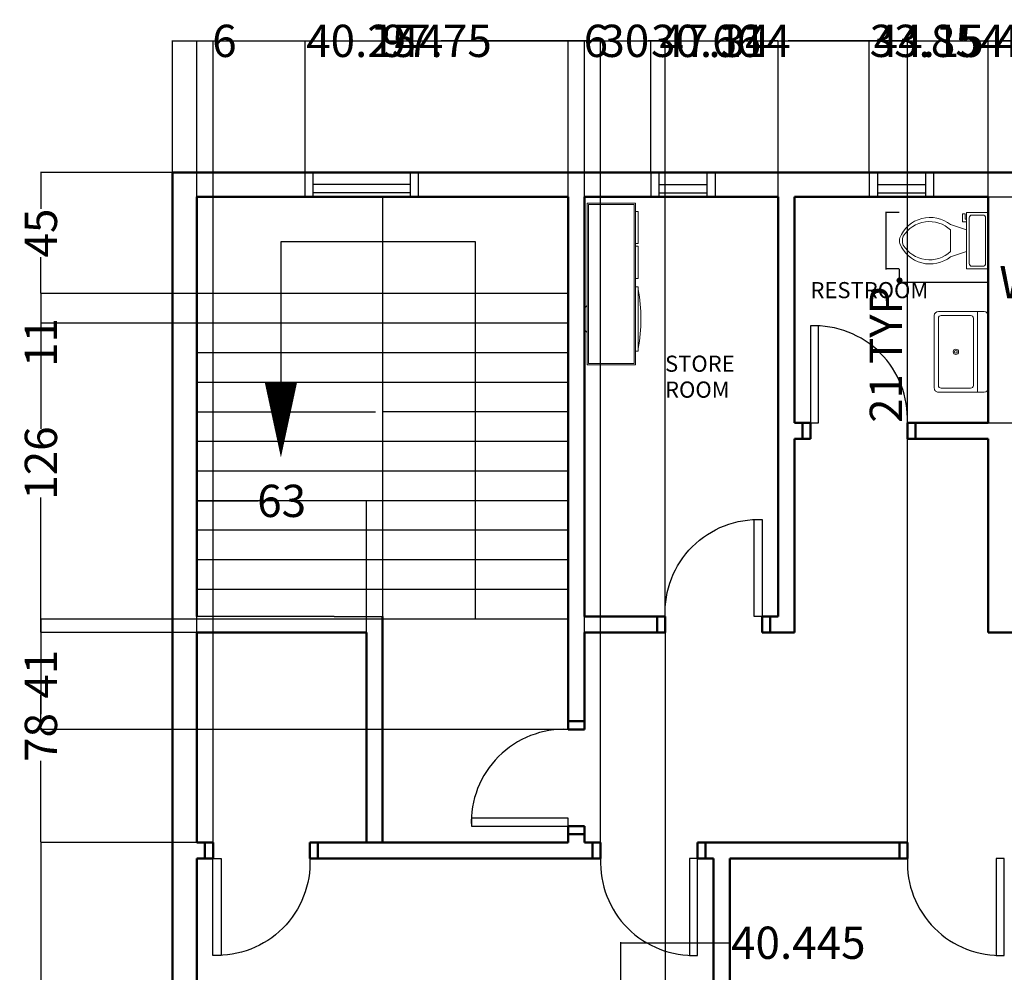
# Model space of a CAD drawing. Units: inches. Extents: x 128 to 1267, y -109 to 1208.
# Tile 6 of 8: x 180 to 546, y 842 to 1196. Entities that reach past the tile are written whole.
import ezdxf

# ---------------------------------------------------------------- set-up
doc = ezdxf.new("R2010")
doc.units = ezdxf.units.IN
doc.header["$MEASUREMENT"] = 0
for name, color, linetype, lineweight in [('A-ANNO-DIMS', 2, 'Continuous', 18), ('A-AREA-IDEN', 3, 'Continuous', 25), ('A-DOOR', 4, 'Continuous', 25), ('A-FLOR-FIXT', 8, 'Continuous', 18), ('A-FLOR-STRS', 2, 'Continuous', 25), ('A-FURN', 8, 'Continuous', 18), ('A-GLAZ', 3, 'Continuous', 25), ('A-WALL', 7, 'Continuous', 50)]:
    doc.layers.add(name, color=color, linetype=linetype, lineweight=lineweight)
doc.styles.get("Standard").update_dxf_attribs({"font": 'arial.ttf'})
doc.dimstyles.get("Standard").update_dxf_attribs({"dimtxt": 12, "dimasz": 0.18, "dimexe": 0.18, "dimexo": 0.0625, "dimgap": 0.09, "dimtad": 0, "dimdec": 1, "dimzin": 0, "dimdsep": 46, "dimlunit": 3, "dimtxsty": 'Standard', "dimcen": 0.09, "dimadec": 0, "dimazin": 0, "dimtfac": 1, "dimtdec": 1, "dimtofl": 0, "dimtmove": 0, "dimatfit": 3, "dimfxl": 1, "dimtolj": 1, "dimtzin": 0, "dimarcsym": 0})

# ---------------------------------------------------------------- blocks, each defined once
blk = doc.blocks.new('Sink-single - 30 in top')
blk.add_line((-15, -3.999996), (15, -3.999996))
for points in [[(-13.5, 0), (13.5, 0)], [(-15, -18.499996), (-15, -1.5)], [(15, -1.5), (15, -18.499996)], [(-13.5, -17.499996), (-13.5, -6.499996)], [(-12.5, -5.499996), (12.5, -5.499996)], [(13.5, -6.499996), (13.5, -17.499996)], [(13.5, -19.999996), (-13.5, -19.999996)], [(12.5, -18.499996), (-12.5, -18.499996)]]:
    blk.add_lwpolyline(points)
for radius in [1, 0.5]:
    blk.add_circle((0, -11.999996), radius)
for centre, radius, start, end in [((-13.5, -1.5), 1.5, 90, 180), ((13.5, -1.5), 1.5, 0, 90), ((-12.5, -6.499996), 1, 90, 180), ((12.5, -6.499996), 1, 0, 90), ((-12.5, -17.499996), 1, 180, 270), ((12.5, -17.499996), 1, 270, 0), ((-13.5, -18.499996), 1.5, 180, 270), ((13.5, -18.499996), 1.5, 270, 0)]:
    blk.add_arc(centre, radius, start, end)
blk = doc.blocks.new('Toilet - top')
for p, q in [((9.5, -6), (9.5, -2)), ((-10, -8.5), (-8, -8.5)), ((-10, -9.5), (-10, -8.5)), ((-7, -9.5), (-10, -9.5)), ((-8, -8.5), (-8, -8)), ((-7, -8), (-7, -9.5)), ((-4, -8), (-6, -14)), ((4, -8), (6, -14)), ((4, -14), (-4, -14))]:
    blk.add_line(p, q)
blk.add_lwpolyline([(10.5, -8), (10.5, 0), (-10.5, 0), (-10.5, -8)], close=True)
for points in [[(-9.5, -2), (-9.5, -6)], [(8.5, -1), (-8.5, -1)], [(-8.5, -7), (8.5, -7)]]:
    blk.add_lwpolyline(points)
for centre, radius, start, end in [((-8.62, -1.88), 0.884, 81.8699, 188.1301), ((8.62, -1.88), 0.884, 351.8699, 98.1301), ((-8.62, -6.12), 0.884, 171.8699, 278.1301), ((8.62, -6.12), 0.884, 261.8699, 8.1301), ((3.52, -21.58), 12.17, 141.4691, 247.9714), ((4.2, -21.82), 11.33, 136.3677, 238.9468), ((-3.52, -21.58), 12.17, 292.0284, 38.5307), ((-4.2, -21.82), 11.33, 301.053, 43.6321), ((0, -27.88), 4, 245.7318, 294.2682), ((0, -29), 4, 254.8605, 285.1395)]:
    blk.add_arc(centre, radius, start, end)
blk = doc.blocks.new('Entertainment Center')
for p, q in [((-4, 0), (-5, -1)), ((4, 0), (-4, 0)), ((5, -1), (4, 0)), ((-17, -19), (-17, -1)), ((-17, -1), (43, -1)), ((-16.5, -18.5), (-16.5, -1.5)), ((-16.5, -1.5), (42.5, -1.5)), ((42.5, -1.5), (42.5, -18.5)), ((43, -1), (43, -19)), ((43, -19), (-17, -19)), ((42.5, -18.5), (-16.5, -18.5)), ((-12, -20), (-12, -19)), ((12, -20), (-12, -20)), ((12, -19), (12, -20)), ((15, -20), (15, -19)), ((27, -20), (15, -20)), ((27, -19), (27, -20)), ((28, -20), (28, -19)), ((40, -20), (28, -20)), ((40, -19), (40, -20))]:
    blk.add_line(p, q)
blk.add_arc((0, 40), 61, 259.6111, 280.3889)
blk = doc.blocks.new('DOOR-900')
blk.add_lwpolyline([(460.06, 187.64), (457.06, 187.64), (457.06, 151.64), (460.06, 151.64)], close=True)
blk.add_arc((458.56, 186.14), 34.53, 177.5104, 272.4896)
blk = doc.blocks.new('WIN-900')
for p, q in [((1102.06, 345.56), (1111.06, 345.56)), ((1102.06, 342.56), (1111.06, 342.56)), ((1103.56, 306.56), (1103.56, 342.56)), ((1106.56, 306.56), (1106.56, 342.56)), ((1111.06, 306.56), (1102.06, 306.56)), ((1111.06, 303.56), (1102.06, 303.56))]:
    blk.add_line(p, q)
blk = doc.blocks.new('WIN-450')
for p, q in [((323.73, 442.64), (323.73, 433.64)), ((326.73, 442.64), (326.73, 433.64)), ((344.73, 433.64), (344.73, 442.64)), ((347.73, 433.64), (347.73, 442.64)), ((326.73, 438.14), (344.73, 438.14)), ((326.73, 435.14), (344.73, 435.14))]:
    blk.add_line(p, q)
blk = doc.blocks.new('*D16')
at = {"layer": 'A-ANNO-DIMS', "color": 0, "lineweight": -2, "transparency": 16777216}
for p, q in [((507.08, 1103.32), (507.08, 1098.25)), ((540.13, 1103.32), (540.13, 1098.25)), ((507.26, 1098.43), (539.95, 1098.43)), ((540.13, 1098.43), (540.31, 1098.43))]:
    blk.add_line(p, q, dxfattribs=at)
at = {"layer": 'A-ANNO-DIMS', "color": 0, "transparency": 16777216}
for points in [[(507.26, 1098.46), (507.26, 1098.4), (507.08, 1098.43)], [(539.95, 1098.46), (539.95, 1098.4), (540.13, 1098.43)]]:
    blk.add_solid(points, dxfattribs=at)
at = {"layer": 'Defpoints', "color": 0, "transparency": 16777216}
for p in [(507.08, 1103.38), (540.13, 1103.38), (540.13, 1098.43)]:
    blk.add_point(p, dxfattribs=at)
at = {"layer": 'A-ANNO-DIMS', "color": 0, "transparency": 16777216, "insert": (586.14, 1098.43), "char_height": 12, "attachment_point": 5}
blk.add_mtext('\\A1;WC 33 TYP.', dxfattribs=at)
blk = doc.blocks.new('*D17')
at = {"layer": 'A-ANNO-DIMS', "color": 0, "lineweight": -2, "transparency": 16777216}
for p, q in [((507.02, 1124.38), (501.94, 1124.38)), ((502.12, 1124.2), (502.12, 1103.56)), ((507.02, 1103.38), (501.94, 1103.38)), ((502.12, 1103.38), (502.12, 1103.2))]:
    blk.add_line(p, q, dxfattribs=at)
at = {"layer": 'A-ANNO-DIMS', "color": 0, "transparency": 16777216}
for points in [[(502.09, 1124.2), (502.15, 1124.2), (502.12, 1124.38)], [(502.09, 1103.56), (502.15, 1103.56), (502.12, 1103.38)]]:
    blk.add_solid(points, dxfattribs=at)
at = {"layer": 'Defpoints', "color": 0, "transparency": 16777216}
for p in [(507.08, 1124.38), (502.12, 1103.38), (507.08, 1103.38)]:
    blk.add_point(p, dxfattribs=at)
at = {"layer": 'A-ANNO-DIMS', "color": 0, "transparency": 16777216, "insert": (502.12, 1073.8), "char_height": 12, "attachment_point": 5, "rotation": 90}
blk.add_mtext('\\A1;21 TYP.', dxfattribs=at)
blk = doc.blocks.new('*D93')
at = {"layer": 'A-ANNO-DIMS', "color": 0, "lineweight": -2, "transparency": 16777216}
for p, q in [((237.13, 664.93), (237.13, 1188.36)), ((237.31, 1188.18), (667.76, 1188.18)), ((1124.95, 1188.18), (694.49, 1188.18)), ((1125.13, 664.93), (1125.13, 1188.36))]:
    blk.add_line(p, q, dxfattribs=at)
at = {"layer": 'A-ANNO-DIMS', "color": 0, "transparency": 16777216}
for points in [[(237.31, 1188.21), (237.31, 1188.15), (237.13, 1188.18)], [(1124.95, 1188.21), (1124.95, 1188.15), (1125.13, 1188.18)]]:
    blk.add_solid(points, dxfattribs=at)
at = {"layer": 'Defpoints', "color": 0, "transparency": 16777216}
for p in [(1125.13, 1188.18), (237.13, 664.87), (1125.13, 664.87)]:
    blk.add_point(p, dxfattribs=at)
at = {"layer": 'A-ANNO-DIMS', "color": 0, "transparency": 16777216, "insert": (681.13, 1188.18), "char_height": 12, "attachment_point": 5}
blk.add_mtext('\\A1;888', dxfattribs=at)
blk = doc.blocks.new('*D97')
at = {"layer": 'A-ANNO-DIMS', "color": 0, "lineweight": -2, "transparency": 16777216}
for p, q in [((246.13, 1130.29), (246.13, 1188.36)), ((246.31, 1188.18), (286.2, 1188.18)), ((286.38, 1139.29), (286.38, 1188.36)), ((286.38, 1188.18), (286.56, 1188.18))]:
    blk.add_line(p, q, dxfattribs=at)
at = {"layer": 'A-ANNO-DIMS', "color": 0, "transparency": 16777216}
for points in [[(246.31, 1188.21), (246.31, 1188.15), (246.13, 1188.18)], [(286.2, 1188.21), (286.2, 1188.15), (286.38, 1188.18)]]:
    blk.add_solid(points, dxfattribs=at)
at = {"layer": 'Defpoints', "color": 0, "transparency": 16777216}
for p in [(286.38, 1188.18), (286.38, 1139.23), (246.13, 1130.23)]:
    blk.add_point(p, dxfattribs=at)
at = {"layer": 'A-ANNO-DIMS', "color": 0, "transparency": 16777216, "insert": (307.18, 1188.18), "char_height": 12, "attachment_point": 5}
blk.add_mtext('\\A1;40.25', dxfattribs=at)
blk = doc.blocks.new('*D98')
at = {"layer": 'A-ANNO-DIMS', "color": 0, "lineweight": -2, "transparency": 16777216}
for p, q in [((286.38, 1139.29), (286.38, 1188.36)), ((286.56, 1188.18), (314.87, 1188.18)), ((383.95, 1188.18), (355.63, 1188.18)), ((384.13, 1130.29), (384.13, 1188.36))]:
    blk.add_line(p, q, dxfattribs=at)
at = {"layer": 'A-ANNO-DIMS', "color": 0, "transparency": 16777216}
for points in [[(286.56, 1188.21), (286.56, 1188.15), (286.38, 1188.18)], [(383.95, 1188.21), (383.95, 1188.15), (384.13, 1188.18)]]:
    blk.add_solid(points, dxfattribs=at)
at = {"layer": 'Defpoints', "color": 0, "transparency": 16777216}
for p in [(384.13, 1188.18), (286.38, 1139.23), (384.13, 1130.23)]:
    blk.add_point(p, dxfattribs=at)
at = {"layer": 'A-ANNO-DIMS', "color": 0, "transparency": 16777216, "insert": (335.25, 1188.18), "char_height": 12, "attachment_point": 5}
blk.add_mtext('\\A1;97.75', dxfattribs=at)
blk = doc.blocks.new('*D99')
at = {"layer": 'A-ANNO-DIMS', "color": 0, "lineweight": -2, "transparency": 16777216}
for p, q in [((384.13, 1130.29), (384.13, 1188.36)), ((384.31, 1188.18), (414.61, 1188.18)), ((414.79, 1139.29), (414.79, 1188.36)), ((414.79, 1188.18), (414.97, 1188.18))]:
    blk.add_line(p, q, dxfattribs=at)
at = {"layer": 'A-ANNO-DIMS', "color": 0, "transparency": 16777216}
for points in [[(384.31, 1188.21), (384.31, 1188.15), (384.13, 1188.18)], [(414.61, 1188.21), (414.61, 1188.15), (414.79, 1188.18)]]:
    blk.add_solid(points, dxfattribs=at)
at = {"layer": 'Defpoints', "color": 0, "transparency": 16777216}
for p in [(414.79, 1188.18), (414.79, 1139.23), (384.13, 1130.23)]:
    blk.add_point(p, dxfattribs=at)
at = {"layer": 'A-ANNO-DIMS', "color": 0, "transparency": 16777216, "insert": (435.3, 1188.18), "char_height": 12, "attachment_point": 5}
blk.add_mtext('\\A1;30.66', dxfattribs=at)
blk = doc.blocks.new('*D100')
at = {"layer": 'A-ANNO-DIMS', "color": 0, "lineweight": -2, "transparency": 16777216}
for p, q in [((414.79, 1139.29), (414.79, 1188.36)), ((414.97, 1188.18), (417.9, 1188.18)), ((461.95, 1188.18), (459.01, 1188.18)), ((462.13, 1130.29), (462.13, 1188.36))]:
    blk.add_line(p, q, dxfattribs=at)
at = {"layer": 'A-ANNO-DIMS', "color": 0, "transparency": 16777216}
for points in [[(414.97, 1188.21), (414.97, 1188.15), (414.79, 1188.18)], [(461.95, 1188.21), (461.95, 1188.15), (462.13, 1188.18)]]:
    blk.add_solid(points, dxfattribs=at)
at = {"layer": 'Defpoints', "color": 0, "transparency": 16777216}
for p in [(462.13, 1188.18), (414.79, 1139.23), (462.13, 1130.23)]:
    blk.add_point(p, dxfattribs=at)
at = {"layer": 'A-ANNO-DIMS', "color": 0, "transparency": 16777216, "insert": (438.46, 1188.18), "char_height": 12, "attachment_point": 5}
blk.add_mtext('\\A1;47.34', dxfattribs=at)
blk = doc.blocks.new('*D101')
at = {"layer": 'A-ANNO-DIMS', "color": 0, "lineweight": -2, "transparency": 16777216}
for p, q in [((462.13, 1130.29), (462.13, 1188.36)), ((462.31, 1188.18), (495.79, 1188.18)), ((495.97, 1139.29), (495.97, 1188.36)), ((495.97, 1188.18), (496.15, 1188.18))]:
    blk.add_line(p, q, dxfattribs=at)
at = {"layer": 'A-ANNO-DIMS', "color": 0, "transparency": 16777216}
for points in [[(462.31, 1188.21), (462.31, 1188.15), (462.13, 1188.18)], [(495.79, 1188.21), (495.79, 1188.15), (495.97, 1188.18)]]:
    blk.add_solid(points, dxfattribs=at)
at = {"layer": 'Defpoints', "color": 0, "transparency": 16777216}
for p in [(495.97, 1188.18), (495.97, 1139.23), (462.13, 1130.23)]:
    blk.add_point(p, dxfattribs=at)
at = {"layer": 'A-ANNO-DIMS', "color": 0, "transparency": 16777216, "insert": (516.53, 1188.18), "char_height": 12, "attachment_point": 5}
blk.add_mtext('\\A1;33.85', dxfattribs=at)
blk = doc.blocks.new('*D102')
at = {"layer": 'A-ANNO-DIMS', "color": 0, "lineweight": -2, "transparency": 16777216}
for p, q in [((495.97, 1139.29), (495.97, 1188.36)), ((496.15, 1188.18), (497.43, 1188.18)), ((539.95, 1188.18), (538.67, 1188.18)), ((540.13, 1130.29), (540.13, 1188.36))]:
    blk.add_line(p, q, dxfattribs=at)
at = {"layer": 'A-ANNO-DIMS', "color": 0, "transparency": 16777216}
for points in [[(496.15, 1188.21), (496.15, 1188.15), (495.97, 1188.18)], [(539.95, 1188.21), (539.95, 1188.15), (540.13, 1188.18)]]:
    blk.add_solid(points, dxfattribs=at)
at = {"layer": 'Defpoints', "color": 0, "transparency": 16777216}
for p in [(540.13, 1188.18), (495.97, 1139.23), (540.13, 1130.23)]:
    blk.add_point(p, dxfattribs=at)
at = {"layer": 'A-ANNO-DIMS', "color": 0, "transparency": 16777216, "insert": (518.05, 1188.18), "char_height": 12, "attachment_point": 5}
blk.add_mtext('\\A1;44.15', dxfattribs=at)
blk = doc.blocks.new('*D103')
at = {"layer": 'A-ANNO-DIMS', "color": 0, "lineweight": -2, "transparency": 16777216}
for p, q in [((540.13, 1130.29), (540.13, 1188.36)), ((540.31, 1188.18), (542.67, 1188.18)), ((586.06, 1188.18), (583.7, 1188.18)), ((586.24, 1139.29), (586.24, 1188.36))]:
    blk.add_line(p, q, dxfattribs=at)
at = {"layer": 'A-ANNO-DIMS', "color": 0, "transparency": 16777216}
for points in [[(540.31, 1188.21), (540.31, 1188.15), (540.13, 1188.18)], [(586.06, 1188.21), (586.06, 1188.15), (586.24, 1188.18)]]:
    blk.add_solid(points, dxfattribs=at)
at = {"layer": 'Defpoints', "color": 0, "transparency": 16777216}
for p in [(586.24, 1188.18), (586.24, 1139.23), (540.13, 1130.23)]:
    blk.add_point(p, dxfattribs=at)
at = {"layer": 'A-ANNO-DIMS', "color": 0, "transparency": 16777216, "insert": (563.19, 1188.18), "char_height": 12, "attachment_point": 5}
blk.add_mtext('\\A1;46.12', dxfattribs=at)
blk = doc.blocks.new('*D126')
at = {"layer": 'A-ANNO-DIMS', "color": 0, "lineweight": -2, "transparency": 16777216}
for p, q in [((246.06, 890.23), (188, 890.23)), ((188.18, 890.05), (188.18, 823.52)), ((188.18, 731.41), (188.18, 797.93)), ((237.06, 731.23), (188, 731.23))]:
    blk.add_line(p, q, dxfattribs=at)
at = {"layer": 'A-ANNO-DIMS', "color": 0, "transparency": 16777216}
for points in [[(188.15, 890.05), (188.21, 890.05), (188.18, 890.23)], [(188.15, 731.41), (188.21, 731.41), (188.18, 731.23)]]:
    blk.add_solid(points, dxfattribs=at)
at = {"layer": 'Defpoints', "color": 0, "transparency": 16777216}
for p in [(188.18, 890.23), (246.13, 890.23), (237.13, 731.23)]:
    blk.add_point(p, dxfattribs=at)
at = {"layer": 'A-ANNO-DIMS', "color": 0, "transparency": 16777216, "insert": (188.18, 810.73), "char_height": 12, "attachment_point": 5, "rotation": 90}
blk.add_mtext('\\A1;159', dxfattribs=at)
blk = doc.blocks.new('*D127')
at = {"layer": 'A-ANNO-DIMS', "color": 0, "lineweight": -2, "transparency": 16777216}
for p, q in [((246.06, 968.23), (188, 968.23)), ((188.18, 968.05), (188.18, 937.87)), ((188.18, 890.41), (188.18, 920.58)), ((246.06, 890.23), (188, 890.23))]:
    blk.add_line(p, q, dxfattribs=at)
at = {"layer": 'A-ANNO-DIMS', "color": 0, "transparency": 16777216}
for points in [[(188.15, 968.05), (188.21, 968.05), (188.18, 968.23)], [(188.15, 890.41), (188.21, 890.41), (188.18, 890.23)]]:
    blk.add_solid(points, dxfattribs=at)
at = {"layer": 'Defpoints', "color": 0, "transparency": 16777216}
for p in [(188.18, 968.23), (246.13, 968.23), (246.13, 890.23)]:
    blk.add_point(p, dxfattribs=at)
at = {"layer": 'A-ANNO-DIMS', "color": 0, "transparency": 16777216, "insert": (188.18, 929.23), "char_height": 12, "attachment_point": 5, "rotation": 90}
blk.add_mtext('\\A1;78', dxfattribs=at)
blk = doc.blocks.new('*D128')
at = {"layer": 'A-ANNO-DIMS', "color": 0, "lineweight": -2, "transparency": 16777216}
for p, q in [((246.06, 1094.23), (188, 1094.23)), ((188.18, 1094.05), (188.18, 1044)), ((188.18, 968.41), (188.18, 1018.45)), ((246.06, 968.23), (188, 968.23))]:
    blk.add_line(p, q, dxfattribs=at)
at = {"layer": 'A-ANNO-DIMS', "color": 0, "transparency": 16777216}
for points in [[(188.15, 1094.05), (188.21, 1094.05), (188.18, 1094.23)], [(188.15, 968.41), (188.21, 968.41), (188.18, 968.23)]]:
    blk.add_solid(points, dxfattribs=at)
at = {"layer": 'Defpoints', "color": 0, "transparency": 16777216}
for p in [(188.18, 1094.23), (246.13, 1094.23), (246.13, 968.23)]:
    blk.add_point(p, dxfattribs=at)
at = {"layer": 'A-ANNO-DIMS', "color": 0, "transparency": 16777216, "insert": (188.18, 1031.23), "char_height": 12, "attachment_point": 5, "rotation": 90}
blk.add_mtext('\\A1;126', dxfattribs=at)
blk = doc.blocks.new('*D129')
at = {"layer": 'A-ANNO-DIMS', "color": 0, "lineweight": -2, "transparency": 16777216}
for p, q in [((237.06, 1139.23), (188, 1139.23)), ((188.18, 1139.05), (188.18, 1125.7)), ((188.18, 1094.41), (188.18, 1107.76)), ((246.06, 1094.23), (188, 1094.23))]:
    blk.add_line(p, q, dxfattribs=at)
at = {"layer": 'A-ANNO-DIMS', "color": 0, "transparency": 16777216}
for points in [[(188.15, 1139.05), (188.21, 1139.05), (188.18, 1139.23)], [(188.15, 1094.41), (188.21, 1094.41), (188.18, 1094.23)]]:
    blk.add_solid(points, dxfattribs=at)
at = {"layer": 'Defpoints', "color": 0, "transparency": 16777216}
for p in [(188.18, 1139.23), (237.13, 1139.23), (246.13, 1094.23)]:
    blk.add_point(p, dxfattribs=at)
at = {"layer": 'A-ANNO-DIMS', "color": 0, "transparency": 16777216, "insert": (188.18, 1116.73), "char_height": 12, "attachment_point": 5, "rotation": 90}
blk.add_mtext('\\A1;45', dxfattribs=at)
blk = doc.blocks.new('*D134')
at = {"layer": 'A-ANNO-DIMS', "color": 0, "lineweight": -2, "transparency": 16777216}
for p, q in [((384.13, 1130.29), (384.13, 1188.36)), ((384.31, 1188.18), (389.95, 1188.18)), ((390.13, 1130.29), (390.13, 1188.36)), ((390.13, 1188.18), (390.31, 1188.18))]:
    blk.add_line(p, q, dxfattribs=at)
at = {"layer": 'A-ANNO-DIMS', "color": 0, "transparency": 16777216}
for points in [[(384.31, 1188.21), (384.31, 1188.15), (384.13, 1188.18)], [(389.95, 1188.21), (389.95, 1188.15), (390.13, 1188.18)]]:
    blk.add_solid(points, dxfattribs=at)
at = {"layer": 'Defpoints', "color": 0, "transparency": 16777216}
for p in [(390.13, 1188.18), (384.13, 1130.23), (390.13, 1130.23)]:
    blk.add_point(p, dxfattribs=at)
at = {"layer": 'A-ANNO-DIMS', "color": 0, "transparency": 16777216, "insert": (394.36, 1188.18), "char_height": 12, "attachment_point": 5}
blk.add_mtext('\\A1;6', dxfattribs=at)
blk = doc.blocks.new('*D135')
at = {"layer": 'A-ANNO-DIMS', "color": 0, "lineweight": -2, "transparency": 16777216}
for p, q in [((540.19, 1130.23), (589.26, 1130.23)), ((589.08, 1130.05), (589.08, 1096.89)), ((589.08, 1046.41), (589.08, 1079.56)), ((540.19, 1046.23), (589.26, 1046.23))]:
    blk.add_line(p, q, dxfattribs=at)
at = {"layer": 'A-ANNO-DIMS', "color": 0, "transparency": 16777216}
for points in [[(589.05, 1130.05), (589.11, 1130.05), (589.08, 1130.23)], [(589.05, 1046.41), (589.11, 1046.41), (589.08, 1046.23)]]:
    blk.add_solid(points, dxfattribs=at)
at = {"layer": 'Defpoints', "color": 0, "transparency": 16777216}
for p in [(540.13, 1130.23), (540.13, 1046.23), (589.08, 1046.23)]:
    blk.add_point(p, dxfattribs=at)
at = {"layer": 'A-ANNO-DIMS', "color": 0, "transparency": 16777216, "insert": (589.08, 1088.23), "char_height": 12, "attachment_point": 5, "rotation": 90}
blk.add_mtext('\\A1;84', dxfattribs=at)
blk = doc.blocks.new('*D136')
at = {"layer": 'A-ANNO-DIMS', "color": 0, "lineweight": -2, "transparency": 16777216}
for p, q in [((384.06, 973.23), (188, 973.23)), ((188.18, 973.05), (188.18, 960.49)), ((188.18, 932.41), (188.18, 944.96)), ((384.06, 932.23), (188, 932.23))]:
    blk.add_line(p, q, dxfattribs=at)
at = {"layer": 'A-ANNO-DIMS', "color": 0, "transparency": 16777216}
for points in [[(188.15, 973.05), (188.21, 973.05), (188.18, 973.23)], [(188.15, 932.41), (188.21, 932.41), (188.18, 932.23)]]:
    blk.add_solid(points, dxfattribs=at)
at = {"layer": 'Defpoints', "color": 0, "transparency": 16777216}
for p in [(384.13, 973.23), (188.18, 932.23), (384.13, 932.23)]:
    blk.add_point(p, dxfattribs=at)
at = {"layer": 'A-ANNO-DIMS', "color": 0, "transparency": 16777216, "insert": (188.18, 952.73), "char_height": 12, "attachment_point": 5, "rotation": 90}
blk.add_mtext('\\A1;41', dxfattribs=at)
blk = doc.blocks.new('*D137')
at = {"layer": 'A-ANNO-DIMS', "color": 0, "lineweight": -2, "transparency": 16777216}
for p, q in [((246.13, 968.29), (246.13, 1017.36)), ((246.31, 1017.18), (268.91, 1017.18)), ((308.95, 1017.18), (286.34, 1017.18)), ((309.13, 968.29), (309.13, 1017.36))]:
    blk.add_line(p, q, dxfattribs=at)
at = {"layer": 'A-ANNO-DIMS', "color": 0, "transparency": 16777216}
for points in [[(246.31, 1017.21), (246.31, 1017.15), (246.13, 1017.18)], [(308.95, 1017.21), (308.95, 1017.15), (309.13, 1017.18)]]:
    blk.add_solid(points, dxfattribs=at)
at = {"layer": 'Defpoints', "color": 0, "transparency": 16777216}
for p in [(309.13, 1017.18), (246.13, 968.23), (309.13, 968.23)]:
    blk.add_point(p, dxfattribs=at)
at = {"layer": 'A-ANNO-DIMS', "color": 0, "transparency": 16777216, "insert": (277.63, 1017.18), "char_height": 12, "attachment_point": 5}
blk.add_mtext('\\A1;63', dxfattribs=at)
blk = doc.blocks.new('*D138')
at = {"layer": 'A-ANNO-DIMS', "color": 0, "lineweight": -2, "transparency": 16777216}
for p, q in [((246.06, 1094.23), (188, 1094.23)), ((188.18, 1094.05), (188.18, 1083.41)), ((246.06, 1083.23), (188, 1083.23)), ((188.18, 1083.23), (188.18, 1083.05))]:
    blk.add_line(p, q, dxfattribs=at)
at = {"layer": 'A-ANNO-DIMS', "color": 0, "transparency": 16777216}
for points in [[(188.15, 1094.05), (188.21, 1094.05), (188.18, 1094.23)], [(188.15, 1083.41), (188.21, 1083.41), (188.18, 1083.23)]]:
    blk.add_solid(points, dxfattribs=at)
at = {"layer": 'Defpoints', "color": 0, "transparency": 16777216}
for p in [(246.13, 1094.23), (188.18, 1083.23), (246.13, 1083.23)]:
    blk.add_point(p, dxfattribs=at)
at = {"layer": 'A-ANNO-DIMS', "color": 0, "transparency": 16777216, "insert": (188.18, 1076.08), "char_height": 12, "attachment_point": 5, "rotation": 90}
blk.add_mtext('\\A1;11', dxfattribs=at)
blk = doc.blocks.new('*D141')
at = {"layer": 'A-ANNO-DIMS', "color": 0, "lineweight": -2, "transparency": 16777216}
for p, q in [((403.68, 804.03), (403.68, 853.1)), ((403.86, 852.92), (443.95, 852.92)), ((444.13, 804.03), (444.13, 853.1)), ((444.13, 852.92), (444.31, 852.92))]:
    blk.add_line(p, q, dxfattribs=at)
at = {"layer": 'A-ANNO-DIMS', "color": 0, "transparency": 16777216}
for points in [[(403.86, 852.95), (403.86, 852.89), (403.68, 852.92)], [(443.95, 852.95), (443.95, 852.89), (444.13, 852.92)]]:
    blk.add_solid(points, dxfattribs=at)
at = {"layer": 'Defpoints', "color": 0, "transparency": 16777216}
for p in [(444.13, 852.92), (403.68, 803.97), (444.13, 803.97)]:
    blk.add_point(p, dxfattribs=at)
at = {"layer": 'A-ANNO-DIMS', "color": 0, "transparency": 16777216, "insert": (469.59, 852.92), "char_height": 12, "attachment_point": 5}
blk.add_mtext('\\A1;40.445', dxfattribs=at)
blk = doc.blocks.new('*D147')
at = {"layer": 'A-ANNO-DIMS', "color": 0, "lineweight": -2, "transparency": 16777216}
for p, q in [((390.13, 968.29), (390.13, 1188.36)), ((390.31, 1188.18), (396.47, 1188.18)), ((419.95, 1188.18), (413.79, 1188.18)), ((420.13, 968.29), (420.13, 1188.36))]:
    blk.add_line(p, q, dxfattribs=at)
at = {"layer": 'A-ANNO-DIMS', "color": 0, "transparency": 16777216}
for points in [[(390.31, 1188.21), (390.31, 1188.15), (390.13, 1188.18)], [(419.95, 1188.21), (419.95, 1188.15), (420.13, 1188.18)]]:
    blk.add_solid(points, dxfattribs=at)
at = {"layer": 'Defpoints', "color": 0, "transparency": 16777216}
for p in [(420.13, 1188.18), (390.13, 968.23), (420.13, 968.23)]:
    blk.add_point(p, dxfattribs=at)
at = {"layer": 'A-ANNO-DIMS', "color": 0, "transparency": 16777216, "insert": (405.13, 1188.18), "char_height": 12, "attachment_point": 5}
blk.add_mtext('\\A1;30', dxfattribs=at)
blk = doc.blocks.new('*D148')
at = {"layer": 'A-ANNO-DIMS', "color": 0, "lineweight": -2, "transparency": 16777216}
for p, q in [((420.13, 968.16), (420.13, 615.74)), ((624.13, 968.16), (624.13, 615.74)), ((420.31, 615.92), (508.7, 615.92)), ((623.95, 615.92), (535.55, 615.92))]:
    blk.add_line(p, q, dxfattribs=at)
at = {"layer": 'A-ANNO-DIMS', "color": 0, "transparency": 16777216}
for points in [[(420.31, 615.95), (420.31, 615.89), (420.13, 615.92)], [(623.95, 615.95), (623.95, 615.89), (624.13, 615.92)]]:
    blk.add_solid(points, dxfattribs=at)
at = {"layer": 'Defpoints', "color": 0, "transparency": 16777216}
for p in [(420.13, 968.23), (624.13, 968.23), (624.13, 615.92)]:
    blk.add_point(p, dxfattribs=at)
at = {"layer": 'A-ANNO-DIMS', "color": 0, "transparency": 16777216, "insert": (522.13, 615.92), "char_height": 12, "attachment_point": 5}
blk.add_mtext('\\A1;204', dxfattribs=at)
blk = doc.blocks.new('*D150')
at = {"layer": 'A-ANNO-DIMS', "color": 0, "lineweight": -2, "transparency": 16777216}
for p, q in [((246.13, 890.29), (246.13, 1188.36)), ((246.31, 1188.18), (251.95, 1188.18)), ((252.13, 890.29), (252.13, 1188.36)), ((252.13, 1188.18), (252.31, 1188.18))]:
    blk.add_line(p, q, dxfattribs=at)
at = {"layer": 'A-ANNO-DIMS', "color": 0, "transparency": 16777216}
for points in [[(246.31, 1188.21), (246.31, 1188.15), (246.13, 1188.18)], [(251.95, 1188.21), (251.95, 1188.15), (252.13, 1188.18)]]:
    blk.add_solid(points, dxfattribs=at)
at = {"layer": 'Defpoints', "color": 0, "transparency": 16777216}
for p in [(252.13, 1188.18), (246.13, 890.23), (252.13, 890.23)]:
    blk.add_point(p, dxfattribs=at)
at = {"layer": 'A-ANNO-DIMS', "color": 0, "transparency": 16777216, "insert": (256.36, 1188.18), "char_height": 12, "attachment_point": 5}
blk.add_mtext('\\A1;6', dxfattribs=at)
blk = doc.blocks.new('*D151')
at = {"layer": 'A-ANNO-DIMS', "color": 0, "lineweight": -2, "transparency": 16777216}
for p, q in [((252.13, 890.29), (252.13, 1188.36)), ((252.31, 1188.18), (311.37, 1188.18)), ((395.95, 1188.18), (336.88, 1188.18)), ((396.13, 890.29), (396.13, 1188.36))]:
    blk.add_line(p, q, dxfattribs=at)
at = {"layer": 'A-ANNO-DIMS', "color": 0, "transparency": 16777216}
for points in [[(252.31, 1188.21), (252.31, 1188.15), (252.13, 1188.18)], [(395.95, 1188.21), (395.95, 1188.15), (396.13, 1188.18)]]:
    blk.add_solid(points, dxfattribs=at)
at = {"layer": 'Defpoints', "color": 0, "transparency": 16777216}
for p in [(396.13, 1188.18), (252.13, 890.23), (396.13, 890.23)]:
    blk.add_point(p, dxfattribs=at)
at = {"layer": 'A-ANNO-DIMS', "color": 0, "transparency": 16777216, "insert": (324.13, 1188.18), "char_height": 12, "attachment_point": 5}
blk.add_mtext('\\A1;144', dxfattribs=at)
blk = doc.blocks.new('*D152')
at = {"layer": 'A-ANNO-DIMS', "color": 0, "lineweight": -2, "transparency": 16777216}
for p, q in [((396.13, 890.29), (396.13, 1188.36)), ((396.31, 1188.18), (440.37, 1188.18)), ((509.95, 1188.18), (465.88, 1188.18)), ((510.13, 890.29), (510.13, 1188.36))]:
    blk.add_line(p, q, dxfattribs=at)
at = {"layer": 'A-ANNO-DIMS', "color": 0, "transparency": 16777216}
for points in [[(396.31, 1188.21), (396.31, 1188.15), (396.13, 1188.18)], [(509.95, 1188.21), (509.95, 1188.15), (510.13, 1188.18)]]:
    blk.add_solid(points, dxfattribs=at)
at = {"layer": 'Defpoints', "color": 0, "transparency": 16777216}
for p in [(510.13, 1188.18), (396.13, 890.23), (510.13, 890.23)]:
    blk.add_point(p, dxfattribs=at)
at = {"layer": 'A-ANNO-DIMS', "color": 0, "transparency": 16777216, "insert": (453.13, 1188.18), "char_height": 12, "attachment_point": 5}
blk.add_mtext('\\A1;114', dxfattribs=at)
blk = doc.blocks.new('*D153')
at = {"layer": 'A-ANNO-DIMS', "color": 0, "lineweight": -2, "transparency": 16777216}
for p, q in [((510.13, 890.29), (510.13, 1188.36)), ((510.31, 1188.18), (528.47, 1188.18)), ((563.95, 1188.18), (545.79, 1188.18)), ((564.13, 890.29), (564.13, 1188.36))]:
    blk.add_line(p, q, dxfattribs=at)
at = {"layer": 'A-ANNO-DIMS', "color": 0, "transparency": 16777216}
for points in [[(510.31, 1188.21), (510.31, 1188.15), (510.13, 1188.18)], [(563.95, 1188.21), (563.95, 1188.15), (564.13, 1188.18)]]:
    blk.add_solid(points, dxfattribs=at)
at = {"layer": 'Defpoints', "color": 0, "transparency": 16777216}
for p in [(564.13, 1188.18), (510.13, 890.23), (564.13, 890.23)]:
    blk.add_point(p, dxfattribs=at)
at = {"layer": 'A-ANNO-DIMS', "color": 0, "transparency": 16777216, "insert": (537.13, 1188.18), "char_height": 12, "attachment_point": 5}
blk.add_mtext('\\A1;54', dxfattribs=at)

msp = doc.modelspace()

# ---------------------------------------------------------------- linework, layer by layer
at = {"layer": 'A-FLOR-STRS'}
for p, q in [((315.1268, 1130.2265), (315.1268, 974.2265)), ((384.1268, 1094.2265), (246.1268, 1094.2265)), ((384.1268, 1083.2265), (246.1268, 1083.2265)), ((384.1268, 1072.2265), (246.1268, 1072.2265)), ((315.1268, 1061.2265), (246.1268, 1061.2265)), ((384.1268, 1061.2265), (315.1268, 1061.2265)), ((312.5162, 1050.0976), (246.1268, 1050.0976)), ((384.1268, 1050.2265), (315.1268, 1050.2265)), ((315.1268, 1039.2265), (246.1268, 1039.2265)), ((384.1268, 1039.2265), (315.1268, 1039.2265)), ((315.1268, 1028.2265), (246.1268, 1028.2265)), ((384.1268, 1028.2265), (315.1268, 1028.2265)), ((315.1268, 1017.2265), (246.1268, 1017.2265)), ((384.1268, 1017.2265), (315.1268, 1017.2265)), ((315.1268, 1006.2265), (246.1268, 1006.2265)), ((384.1268, 1006.2265), (315.1268, 1006.2265)), ((315.1268, 995.2265), (246.1268, 995.2265)), ((384.1268, 995.2265), (315.1268, 995.2265)), ((315.1268, 984.2265), (246.1268, 984.2265)), ((384.1268, 984.2265), (315.1268, 984.2265)), ((297.1268, 974.2265), (246.1268, 974.2265)), ((297.1268, 974.2265), (315.1268, 974.2265)), ((384.1268, 973.2265), (315.1268, 973.2265))]:
    msp.add_line(p, q, dxfattribs=at)
msp.add_lwpolyline([(349.6268, 973.2265), (349.6268, 1113.4165), (277.3594, 1113.4165), (277.3594, 1061.2265)], dxfattribs=at)
msp.add_lwpolyline([(277.3594, 1061.2265, 12, 0, 0), (277.3594, 1033.3075, 0, 0, 0)], format="xyseb", dxfattribs=at)
at = {"layer": 'A-WALL'}
for p, q in [((516.9736, 1139.2265), (498.9736, 1139.2265)), ((246.1268, 1130.2265), (246.1268, 974.2265)), ((246.1268, 1130.2265), (246.1268, 974.2265)), ((384.1268, 1130.2265), (246.1268, 1130.2265)), ((384.1268, 932.2265), (384.1268, 1130.2265)), ((462.1268, 1130.2265), (390.1268, 1130.2265)), ((390.1268, 974.2265), (390.1268, 1130.2265)), ((462.1268, 974.2265), (462.1268, 1130.2265)), ((540.1268, 1130.2265), (468.1268, 1130.2265)), ((468.1268, 1046.2265), (468.1268, 1130.2265)), ((498.9736, 1130.2265), (516.9736, 1130.2265)), ((540.1268, 1046.2265), (540.1268, 1130.2265)), ((474.1268, 1046.2265), (468.1268, 1046.2265)), ((471.1268, 1046.2265), (471.1268, 1040.2265)), ((474.1268, 1046.2265), (474.1268, 1040.2265)), ((540.1268, 1046.2265), (510.1268, 1046.2265)), ((510.1268, 1046.2265), (510.1268, 1040.2265)), ((513.1268, 1046.2265), (513.1268, 1040.2265)), ((468.1268, 968.2265), (468.1268, 1040.2265)), ((474.1268, 1040.2265), (468.1268, 1040.2265)), ((540.1268, 1040.2265), (510.1268, 1040.2265)), ((540.1268, 968.2265), (540.1268, 1040.2265)), ((315.1268, 974.2265), (315.1268, 890.2265)), ((420.1268, 974.2265), (390.1268, 974.2265)), ((417.1268, 974.2265), (417.1268, 968.2265)), ((420.1268, 974.2265), (420.1268, 968.2265)), ((462.1268, 974.2265), (456.1268, 974.2265)), ((456.1268, 974.2265), (456.1268, 968.2265)), ((459.1268, 974.2265), (459.1268, 968.2265)), ((246.1268, 968.2265), (246.1268, 890.2265)), ((246.1268, 968.2265), (246.1268, 890.2265)), ((309.1268, 968.2265), (246.1268, 968.2265)), ((309.1268, 968.2265), (309.1268, 890.2265)), ((420.1268, 968.2265), (390.1268, 968.2265)), ((390.1268, 932.2265), (390.1268, 968.2265)), ((468.1268, 968.2265), (456.1268, 968.2265)), ((624.1268, 968.2265), (540.1268, 968.2265)), ((384.1268, 935.2265), (390.1268, 935.2265)), ((384.1268, 932.2265), (390.1268, 932.2265)), ((384.1268, 890.2265), (384.1268, 896.2265)), ((384.1268, 896.2265), (390.1268, 896.2265)), ((384.1268, 893.2265), (390.1268, 893.2265)), ((390.1268, 890.2265), (390.1268, 896.2265)), ((246.1268, 890.2265), (252.1268, 890.2265)), ((249.1268, 884.2265), (249.1268, 890.2265)), ((252.1268, 884.2265), (252.1268, 890.2265)), ((288.1268, 884.2265), (288.1268, 890.2265)), ((288.1268, 890.2265), (384.1268, 890.2265)), ((291.1268, 884.2265), (291.1268, 890.2265)), ((390.1268, 890.2265), (396.1268, 890.2265)), ((393.1268, 884.2265), (393.1268, 890.2265)), ((396.1268, 884.2265), (396.1268, 890.2265)), ((432.1268, 884.2265), (432.1268, 890.2265)), ((432.1268, 890.2265), (510.1268, 890.2265)), ((435.1268, 884.2265), (435.1268, 890.2265)), ((507.1268, 884.2265), (507.1268, 890.2265)), ((510.1268, 884.2265), (510.1268, 890.2265)), ((246.1268, 884.2265), (252.1268, 884.2265)), ((246.1268, 884.2265), (246.1268, 740.2265)), ((288.1268, 884.2265), (396.1268, 884.2265)), ((432.1268, 884.2265), (438.1268, 884.2265)), ((438.1268, 884.2265), (438.1268, 809.9714)), ((444.1268, 884.2265), (444.1268, 803.9714)), ((444.1268, 884.2265), (510.1268, 884.2265))]:
    msp.add_line(p, q, dxfattribs=at)
msp.add_lwpolyline([(1110.1268, 731.2265), (1125.1268, 731.2265), (1125.1268, 1139.2265), (237.1268, 1139.2265), (237.1268, 731.2265), (1038.1268, 731.2265)], dxfattribs=at)

# ---------------------------------------------------------------- block references
at = {"layer": 'A-DOOR'}
for p, rotation in [((934.1828, 1233.8664), 180), ((196.4868, 1356.2825), 270)]:
    msp.add_blockref('DOOR-900', p, dxfattribs=dict(at, rotation=rotation))
at = {"layer": 'A-DOOR', "extrusion": (0, 0, -1), "zscale": -1, "rotation": 180}
msp.add_blockref('DOOR-900', (3.9293, 1161.8664), dxfattribs=at)
at = {"layer": 'A-DOOR', "extrusion": (0, 0, -1), "zscale": -1}
msp.add_blockref('DOOR-900', (-712.1828, 696.5866), dxfattribs=at)
at = {"layer": 'A-DOOR'}
for p in [(-27.9293, 696.5866), (86.0707, 696.5866)]:
    msp.add_blockref('DOOR-900', p, dxfattribs=at)
at = {"layer": 'A-FLOR-FIXT', "rotation": 270}
for name, p in [('Toilet - top', (540.1268, 1113.8829)), ('Sink-single - 30 in top', (540.1268, 1072.5736))]:
    msp.add_blockref(name, p, dxfattribs=at)
at = {"layer": 'A-FURN', "rotation": 90}
msp.add_blockref('Entertainment Center', (390.1268, 1084.8014), dxfattribs=at)
at = {"layer": 'A-GLAZ', "rotation": 90.00000000000108}
msp.add_blockref('WIN-900', (631.9409, 28.1705), dxfattribs=at)
at = {"layer": 'A-GLAZ'}
for p in [(91.0578, 696.5866), (172.2436, 696.5866)]:
    msp.add_blockref('WIN-450', p, dxfattribs=at)

# ---------------------------------------------------------------- texts
at = {"layer": 'A-AREA-IDEN'}
for s, p in [('RESTROOM', (474.0913, 1092.5172)), ('STORE ', (420.0722, 1065.1724)), ('ROOM', (420.0722, 1055.5339))]:
    msp.add_text(s, height=6, dxfattribs=at).set_placement(p)

# ---------------------------------------------------------------- dimensions: what is measured, and where the dimension line sits
at = {"layer": 'A-ANNO-DIMS'}
for base, p1, p2, override, picture, middle in [((1125.1268, 1188.1765), (237.1268, 664.8687), (1125.1268, 664.8687), {"dimdec": 0, "dimlfac": 1, "dimrnd": 0, "dimzin": 0, "dimdsep": 46, "dimlunit": 2}, '*D93', (681.1268, 1188.1765)), ((286.3786, 1188.1765), (246.1268, 1130.2265), (286.3786, 1139.2265), {"dimdec": 2, "dimlfac": 1, "dimrnd": 0, "dimzin": 0, "dimdsep": 46, "dimlunit": 2}, '*D97', (307.182, 1188.1765)), ((252.1268, 1188.1765), (246.1268, 890.2265), (252.1268, 890.2265), {"dimdec": 0, "dimlfac": 1, "dimrnd": 0, "dimzin": 0, "dimdsep": 46, "dimlunit": 2}, '*D150', (256.3586, 1188.1765)), ((396.1268, 1188.1765), (252.1268, 890.2265), (396.1268, 890.2265), {"dimdec": 0, "dimlfac": 1, "dimrnd": 0, "dimzin": 0, "dimdsep": 46, "dimlunit": 2}, '*D151', (324.1268, 1188.1765)), ((384.1268, 1188.1765), (286.3786, 1139.2265), (384.1268, 1130.2265), {"dimdec": 2, "dimlfac": 1, "dimrnd": 0, "dimzin": 0, "dimdsep": 46, "dimlunit": 2}, '*D98', (335.2527, 1188.1765)), ((414.7879, 1188.1765), (384.1268, 1130.2265), (414.7879, 1139.2265), {"dimdec": 2, "dimlfac": 1, "dimrnd": 0, "dimzin": 0, "dimdsep": 46, "dimlunit": 2}, '*D99', (435.2966, 1188.1765)), ((390.1268, 1188.1765), (384.1268, 1130.2265), (390.1268, 1130.2265), {"dimdec": 0, "dimlfac": 1, "dimrnd": 0, "dimzin": 0, "dimdsep": 46, "dimlunit": 2}, '*D134', (394.3586, 1188.1765)), ((420.1268, 1188.1765), (390.1268, 968.2265), (420.1268, 968.2265), {"dimdec": 0, "dimlfac": 1, "dimrnd": 0, "dimzin": 0, "dimdsep": 46, "dimlunit": 2}, '*D147', (405.1268, 1188.1765)), ((510.1268, 1188.1765), (396.1268, 890.2265), (510.1268, 890.2265), {"dimdec": 0, "dimlfac": 1, "dimrnd": 0, "dimzin": 0, "dimdsep": 46, "dimlunit": 2}, '*D152', (453.1268, 1188.1765)), ((462.1268, 1188.1765), (414.7879, 1139.2265), (462.1268, 1130.2265), {"dimdec": 2, "dimlfac": 1, "dimrnd": 0, "dimzin": 0, "dimdsep": 46, "dimlunit": 2}, '*D100', (438.4573, 1188.1765)), ((495.9736, 1188.1765), (462.1268, 1130.2265), (495.9736, 1139.2265), {"dimdec": 2, "dimlfac": 1, "dimrnd": 0, "dimzin": 0, "dimdsep": 46, "dimlunit": 2}, '*D101', (516.5315, 1188.1765)), ((540.1268, 1188.1765), (495.9736, 1139.2265), (540.1268, 1130.2265), {"dimdec": 2, "dimlfac": 1, "dimrnd": 0, "dimzin": 0, "dimdsep": 46, "dimlunit": 2}, '*D102', (518.0502, 1188.1765)), ((564.1268, 1188.1765), (510.1268, 890.2265), (564.1268, 890.2265), {"dimdec": 0, "dimlfac": 1, "dimrnd": 0, "dimzin": 0, "dimdsep": 46, "dimlunit": 2}, '*D153', (537.1268, 1188.1765)), ((586.2442, 1188.1765), (540.1268, 1130.2265), (586.2442, 1139.2265), {"dimdec": 2, "dimlfac": 1, "dimrnd": 0, "dimzin": 0, "dimdsep": 46, "dimlunit": 2}, '*D103', (563.1855, 1188.1765)), ((624.1268, 615.9187), (420.1268, 968.2265), (624.1268, 968.2265), {"dimdec": 0, "dimlfac": 1, "dimrnd": 0, "dimzin": 0, "dimdsep": 46, "dimlunit": 2}, '*D148', (522.1268, 615.9187)), ((444.1268, 852.9214), (403.6821, 803.9714), (444.1268, 803.9714), {"dimdec": 3, "dimlfac": 1, "dimrnd": 0, "dimzin": 0, "dimdsep": 46, "dimlunit": 2}, '*D141', (469.5919, 852.9214))]:
    dim = msp.add_linear_dim(base=base, p1=p1, p2=p2, dimstyle='Standard', override=override, dxfattribs=at)
    dim.commit()
    dim.dimension.update_dxf_attribs({"geometry": picture, "text_midpoint": middle})
for base, p1, p2, angle, picture, middle in [((188.1768, 1139.2265), (246.1268, 1094.2265), (237.1268, 1139.2265), 90, '*D129', (188.1768, 1116.7265)), ((589.0768, 1046.2265), (540.1268, 1130.2265), (540.1268, 1046.2265), 270, '*D135', (589.0768, 1088.2265)), ((188.1768, 1094.2265), (246.1268, 968.2265), (246.1268, 1094.2265), 90, '*D128', (188.1768, 1031.2265)), ((188.1768, 1083.2265), (246.1268, 1094.2265), (246.1268, 1083.2265), 90, '*D138', (188.1768, 1076.0847)), ((309.1268, 1017.1765), (246.1268, 968.2265), (309.1268, 968.2265), 0, '*D137', (277.6268, 1017.1765)), ((188.1768, 932.2265), (384.1268, 973.2265), (384.1268, 932.2265), 90, '*D136', (188.1768, 952.7265)), ((188.1768, 968.2265), (246.1268, 890.2265), (246.1268, 968.2265), 90, '*D127', (188.1768, 929.2265)), ((188.1768, 890.2265), (237.1268, 731.2265), (246.1268, 890.2265), 90, '*D126', (188.1768, 810.7265))]:
    dim = msp.add_linear_dim(base=base, p1=p1, p2=p2, angle=angle, dimstyle='Standard', override={"dimdec": 0, "dimlfac": 1, "dimrnd": 0, "dimzin": 0, "dimdsep": 46, "dimlunit": 2}, dxfattribs=at)
    dim.commit()
    dim.dimension.update_dxf_attribs({"geometry": picture, "text_midpoint": middle})
dim = msp.add_linear_dim(base=(502.1236, 1103.3829), p1=(507.0805, 1124.3829), p2=(507.0805, 1103.3829), angle=270, text='<> TYP.', dimstyle='Standard', override={"dimdec": 0, "dimrnd": 0, "dimzin": 0, "dimlunit": 2}, dxfattribs=at)
dim.commit()
dim.dimension.update_dxf_attribs({"geometry": '*D17', "text_midpoint": (502.1236, 1073.8046)})
dim = msp.add_linear_dim(base=(540.1268, 1098.426), p1=(507.0805, 1103.3829), p2=(540.1268, 1103.3829), text='WC <> TYP.', dimstyle='Standard', override={"dimdec": 0, "dimrnd": 0, "dimzin": 0, "dimlunit": 2}, dxfattribs=at)
dim.commit()
dim.dimension.update_dxf_attribs({"geometry": '*D16', "text_midpoint": (586.1416, 1098.426)})

doc.saveas('drawing.dxf')
